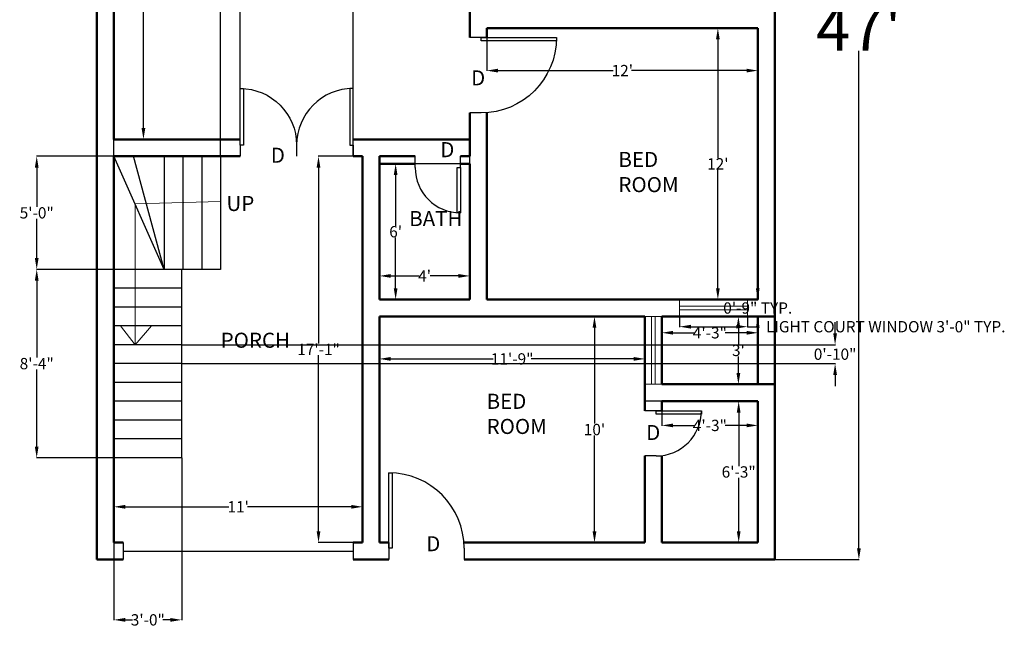
# Model space of a CAD drawing. Units: inches. Extents: x -251 to 272, y 511 to 1173.
# Tile 1 of 2: x -251 to 272, y 511 to 834. Entities that reach past the tile are written whole.
import ezdxf

# ---------------------------------------------------------------- set-up
doc = ezdxf.new("R2010")
doc.units = ezdxf.units.IN
doc.header["$MEASUREMENT"] = 0
doc.layers.get('0').update_dxf_attribs({"color": 3})
for name, color, linetype, lineweight in [('A-ANNO-SYMB', 20, 'Continuous', 18), ('A-AREA-IDEN', 20, 'Continuous', 25), ('A-FLOR', 7, 'Continuous', 25), ('A-WALL', 7, 'Continuous', 50), ('dim', 2, 'Continuous', 18), ('door', 1, 'Continuous', 25), ('stair', 94, 'Continuous', 25), ('text', 20, 'Continuous', 18), ('window', 6, 'Continuous', 18)]:
    doc.layers.add(name, color=color, linetype=linetype, lineweight=lineweight)
doc.styles.get("Standard").update_dxf_attribs({"font": 'arial.ttf'})
doc.dimstyles.get("Standard").update_dxf_attribs({"dimtxt": 6, "dimasz": 6, "dimexe": 0.18, "dimexo": 0.0625, "dimgap": 0.09, "dimtad": 0, "dimtih": 1, "dimtoh": 1, "dimdec": 0, "dimzin": 0, "dimdsep": 46, "dimlunit": 3, "dimtxsty": 'Standard', "dimcen": 0.09, "dimadec": 0, "dimazin": 0, "dimtfac": 1, "dimtdec": 0, "dimtofl": 0, "dimtmove": 0, "dimatfit": 3, "dimfxl": 1, "dimtolj": 1, "dimtzin": 0, "dimarcsym": 0})

# ---------------------------------------------------------------- blocks, each defined once
blk = doc.blocks.new('*U18')
for p, q in [((0, 0), (0, 6)), ((40, 0), (40, 6))]:
    blk.add_line(p, q)
blk.add_lwpolyline([(0, 0), (0, -40), (1.75, -40), (1.75, 0)], close=True)
blk.add_arc((0, 0), 40, 270, 0)
blk = doc.blocks.new('*D21')
at = {"layer": 'Defpoints', "color": 0, "transparency": 16777216}
for p in [(141.31, 829.09), (120.04, 685.09), (141.31, 685.09)]:
    blk.add_point(p, dxfattribs=at)
at = {"layer": 'dim', "color": 0, "lineweight": -2, "transparency": 16777216}
for p, q in [((141.25, 829.09), (119.86, 829.09)), ((120.04, 823.09), (120.04, 760.19)), ((120.04, 691.09), (120.04, 753.99)), ((141.25, 685.09), (119.86, 685.09))]:
    blk.add_line(p, q, dxfattribs=at)
at = {"layer": 'dim', "color": 0, "transparency": 16777216}
for points in [[(119.04, 823.09), (121.04, 823.09), (120.04, 829.09)], [(119.04, 691.09), (121.04, 691.09), (120.04, 685.09)]]:
    blk.add_solid(points, dxfattribs=at)
at = {"layer": 'dim', "color": 0, "transparency": 16777216, "insert": (120.04, 757.09), "char_height": 6, "attachment_point": 5}
blk.add_mtext("\\A1;12'", dxfattribs=at)
blk = doc.blocks.new('*D22')
at = {"layer": 'Defpoints', "color": 0, "transparency": 16777216}
for p in [(-2.69, 829.09), (141.31, 829.09), (-2.69, 806.58)]:
    blk.add_point(p, dxfattribs=at)
at = {"layer": 'dim', "color": 0, "lineweight": -2, "transparency": 16777216}
for p, q in [((-2.69, 829.02), (-2.69, 806.4)), ((141.31, 829.02), (141.31, 806.4)), ((3.31, 806.58), (64.41, 806.58)), ((135.31, 806.58), (74.21, 806.58))]:
    blk.add_line(p, q, dxfattribs=at)
at = {"layer": 'dim', "color": 0, "transparency": 16777216}
for points in [[(3.31, 807.58), (3.31, 805.58), (-2.69, 806.58)], [(135.31, 807.58), (135.31, 805.58), (141.31, 806.58)]]:
    blk.add_solid(points, dxfattribs=at)
at = {"layer": 'dim', "color": 0, "transparency": 16777216, "insert": (69.31, 806.58), "char_height": 6, "attachment_point": 5}
blk.add_mtext("\\A1;12'", dxfattribs=at)
blk = doc.blocks.new('*U23')
for p, q in [((0, 0), (0, -6)), ((24, 0), (24, -6))]:
    blk.add_line(p, q)
blk.add_lwpolyline([(0, 0), (0, 24), (1.75, 24), (1.75, 0)], close=True)
blk.add_arc((0, 0), 24, 0, 90)
blk = doc.blocks.new('*U24')
for p, q in [((-24, 0), (-24, 6)), ((0, 0), (0, 6))]:
    blk.add_line(p, q)
blk.add_lwpolyline([(0, 0), (0, -24), (-1.75, -24), (-1.75, 0)], close=True)
blk.add_arc((0, 0), 24, 180, 270)
blk = doc.blocks.new('*D25')
at = {"layer": 'Defpoints', "color": 0, "transparency": 16777216}
for p in [(-14.19, 757.09), (-51.07, 685.09), (-11.69, 685.09)]:
    blk.add_point(p, dxfattribs=at)
at = {"layer": 'dim', "color": 0, "lineweight": -2, "transparency": 16777216}
for p, q in [((-14.25, 757.09), (-51.25, 757.09)), ((-51.07, 751.09), (-51.07, 724.24)), ((-51.07, 691.09), (-51.07, 717.93)), ((-11.75, 685.09), (-51.25, 685.09))]:
    blk.add_line(p, q, dxfattribs=at)
at = {"layer": 'dim', "color": 0, "transparency": 16777216}
for points in [[(-52.07, 751.09), (-50.07, 751.09), (-51.07, 757.09)], [(-52.07, 691.09), (-50.07, 691.09), (-51.07, 685.09)]]:
    blk.add_solid(points, dxfattribs=at)
at = {"layer": 'dim', "color": 0, "transparency": 16777216, "insert": (-51.07, 721.09), "char_height": 6, "attachment_point": 5}
blk.add_mtext("\\A1;6'", dxfattribs=at)
blk = doc.blocks.new('*D26')
at = {"layer": 'Defpoints', "color": 0, "transparency": 16777216}
for p in [(-11.69, 697.62), (-59.69, 685.09), (-11.69, 685.09)]:
    blk.add_point(p, dxfattribs=at)
at = {"layer": 'dim', "color": 0, "lineweight": -2, "transparency": 16777216}
for p, q in [((-59.69, 685.15), (-59.69, 697.8)), ((-53.69, 697.62), (-38.66, 697.62)), ((-17.69, 697.62), (-32.72, 697.62)), ((-11.69, 685.15), (-11.69, 697.8))]:
    blk.add_line(p, q, dxfattribs=at)
at = {"layer": 'dim', "color": 0, "transparency": 16777216}
for points in [[(-53.69, 698.62), (-53.69, 696.62), (-59.69, 697.62)], [(-17.69, 698.62), (-17.69, 696.62), (-11.69, 697.62)]]:
    blk.add_solid(points, dxfattribs=at)
at = {"layer": 'dim', "color": 0, "transparency": 16777216, "insert": (-35.69, 697.62), "char_height": 6, "attachment_point": 5}
blk.add_mtext("\\A1;4'", dxfattribs=at)
blk = doc.blocks.new('*D27')
at = {"layer": 'Defpoints', "color": 0, "transparency": 16777216}
for p in [(141.31, 676.09), (130.96, 640.09), (141.31, 640.09)]:
    blk.add_point(p, dxfattribs=at)
at = {"layer": 'dim', "color": 0, "lineweight": -2, "transparency": 16777216}
for p, q in [((141.25, 676.09), (130.78, 676.09)), ((130.96, 670.09), (130.96, 661.24)), ((130.96, 646.09), (130.96, 654.93)), ((141.25, 640.09), (130.78, 640.09))]:
    blk.add_line(p, q, dxfattribs=at)
at = {"layer": 'dim', "color": 0, "transparency": 16777216}
for points in [[(129.96, 670.09), (131.96, 670.09), (130.96, 676.09)], [(129.96, 646.09), (131.96, 646.09), (130.96, 640.09)]]:
    blk.add_solid(points, dxfattribs=at)
at = {"layer": 'dim', "color": 0, "transparency": 16777216, "insert": (130.96, 658.09), "char_height": 6, "attachment_point": 5}
blk.add_mtext("\\A1;3'", dxfattribs=at)
blk = doc.blocks.new('*D28')
at = {"layer": 'Defpoints', "color": 0, "transparency": 16777216}
for p in [(90.31, 676.09), (141.31, 676.09), (141.31, 667.45)]:
    blk.add_point(p, dxfattribs=at)
at = {"layer": 'dim', "color": 0, "lineweight": -2, "transparency": 16777216}
for p, q in [((90.31, 676.02), (90.31, 667.27)), ((141.31, 676.02), (141.31, 667.27)), ((96.31, 667.45), (107.63, 667.45)), ((135.31, 667.45), (124, 667.45))]:
    blk.add_line(p, q, dxfattribs=at)
at = {"layer": 'dim', "color": 0, "transparency": 16777216}
for points in [[(96.31, 668.45), (96.31, 666.45), (90.31, 667.45)], [(135.31, 668.45), (135.31, 666.45), (141.31, 667.45)]]:
    blk.add_solid(points, dxfattribs=at)
at = {"layer": 'dim', "color": 0, "transparency": 16777216, "insert": (115.81, 667.45), "char_height": 6, "attachment_point": 5}
blk.add_mtext('\\A1;4\'-3"', dxfattribs=at)
blk = doc.blocks.new('*D29')
at = {"layer": 'Defpoints', "color": 0, "transparency": 16777216}
for p in [(141.31, 631.09), (131.11, 556.09), (141.31, 556.09)]:
    blk.add_point(p, dxfattribs=at)
at = {"layer": 'dim', "color": 0, "lineweight": -2, "transparency": 16777216}
for p, q in [((141.25, 631.09), (130.93, 631.09)), ((131.11, 625.09), (131.11, 596.74)), ((131.11, 562.09), (131.11, 590.43)), ((141.25, 556.09), (130.93, 556.09))]:
    blk.add_line(p, q, dxfattribs=at)
at = {"layer": 'dim', "color": 0, "transparency": 16777216}
for points in [[(130.11, 625.09), (132.11, 625.09), (131.11, 631.09)], [(130.11, 562.09), (132.11, 562.09), (131.11, 556.09)]]:
    blk.add_solid(points, dxfattribs=at)
at = {"layer": 'dim', "color": 0, "transparency": 16777216, "insert": (131.11, 593.59), "char_height": 6, "attachment_point": 5}
blk.add_mtext('\\A1;6\'-3"', dxfattribs=at)
blk = doc.blocks.new('*D30')
at = {"layer": 'Defpoints', "color": 0, "transparency": 16777216}
for p in [(90.31, 631.09), (141.31, 631.09), (141.31, 618.28)]:
    blk.add_point(p, dxfattribs=at)
at = {"layer": 'dim', "color": 0, "lineweight": -2, "transparency": 16777216}
for p, q in [((90.31, 631.02), (90.31, 618.1)), ((141.31, 631.02), (141.31, 618.1)), ((96.31, 618.28), (107.63, 618.28)), ((135.31, 618.28), (124, 618.28))]:
    blk.add_line(p, q, dxfattribs=at)
at = {"layer": 'dim', "color": 0, "transparency": 16777216}
for points in [[(96.31, 619.28), (96.31, 617.28), (90.31, 618.28)], [(135.31, 619.28), (135.31, 617.28), (141.31, 618.28)]]:
    blk.add_solid(points, dxfattribs=at)
at = {"layer": 'dim', "color": 0, "transparency": 16777216, "insert": (115.81, 618.28), "char_height": 6, "attachment_point": 5}
blk.add_mtext('\\A1;4\'-3"', dxfattribs=at)
blk = doc.blocks.new('*U8')
for p, q in [((0, 0), (0, -6)), ((40, 0), (40, -6))]:
    blk.add_line(p, q)
blk.add_lwpolyline([(0, 0), (0, 40), (1.75, 40), (1.75, 0)], close=True)
blk.add_arc((0, 0), 40, 0, 90)
blk = doc.blocks.new('*D31')
at = {"layer": 'Defpoints', "color": 0, "transparency": 16777216}
for p in [(65.76, 676.09), (54.53, 556.09), (65.76, 556.09)]:
    blk.add_point(p, dxfattribs=at)
at = {"layer": 'dim', "color": 0, "lineweight": -2, "transparency": 16777216}
for p, q in [((65.7, 676.09), (54.35, 676.09)), ((54.53, 670.09), (54.53, 619.24)), ((54.53, 562.09), (54.53, 612.93)), ((65.7, 556.09), (54.35, 556.09))]:
    blk.add_line(p, q, dxfattribs=at)
at = {"layer": 'dim', "color": 0, "transparency": 16777216}
for points in [[(53.53, 670.09), (55.53, 670.09), (54.53, 676.09)], [(53.53, 562.09), (55.53, 562.09), (54.53, 556.09)]]:
    blk.add_solid(points, dxfattribs=at)
at = {"layer": 'dim', "color": 0, "transparency": 16777216, "insert": (54.53, 616.09), "char_height": 6, "attachment_point": 5}
blk.add_mtext("\\A1;10'", dxfattribs=at)
blk = doc.blocks.new('*D32')
at = {"layer": 'Defpoints', "color": 0, "transparency": 16777216}
for p in [(-59.69, 676.09), (81.31, 676.09), (81.31, 653.59)]:
    blk.add_point(p, dxfattribs=at)
at = {"layer": 'dim', "color": 0, "lineweight": -2, "transparency": 16777216}
for p, q in [((-59.69, 676.02), (-59.69, 653.41)), ((81.31, 676.02), (81.31, 653.41)), ((-53.69, 653.59), (0.7, 653.59)), ((75.31, 653.59), (20.93, 653.59))]:
    blk.add_line(p, q, dxfattribs=at)
at = {"layer": 'dim', "color": 0, "transparency": 16777216}
for points in [[(-53.69, 654.59), (-53.69, 652.59), (-59.69, 653.59)], [(75.31, 654.59), (75.31, 652.59), (81.31, 653.59)]]:
    blk.add_solid(points, dxfattribs=at)
at = {"layer": 'dim', "color": 0, "transparency": 16777216, "insert": (10.81, 653.59), "char_height": 6, "attachment_point": 5}
blk.add_mtext('\\A1;11\'-9"', dxfattribs=at)
blk = doc.blocks.new('*U33')
for p, q in [((-30, 0), (-30, -6)), ((0, 0), (0, -6))]:
    blk.add_line(p, q)
blk.add_lwpolyline([(0, 0), (0, 30), (-1.75, 30), (-1.75, 0)], close=True)
blk.add_arc((0, 0), 30, 90, 180)
blk = doc.blocks.new('*D34')
at = {"layer": 'Defpoints', "color": 0, "transparency": 16777216}
for p in [(-71.19, 761.09), (-92.03, 556.09), (-71.19, 556.09)]:
    blk.add_point(p, dxfattribs=at)
at = {"layer": 'dim', "color": 0, "lineweight": -2, "transparency": 16777216}
for p, q in [((-71.25, 761.09), (-92.21, 761.09)), ((-92.03, 755.09), (-92.03, 661.69)), ((-92.03, 562.09), (-92.03, 655.49)), ((-71.25, 556.09), (-92.21, 556.09))]:
    blk.add_line(p, q, dxfattribs=at)
at = {"layer": 'dim', "color": 0, "transparency": 16777216}
for points in [[(-93.03, 755.09), (-91.03, 755.09), (-92.03, 761.09)], [(-93.03, 562.09), (-91.03, 562.09), (-92.03, 556.09)]]:
    blk.add_solid(points, dxfattribs=at)
at = {"layer": 'dim', "color": 0, "transparency": 16777216, "insert": (-92.03, 658.59), "char_height": 6, "attachment_point": 5}
blk.add_mtext('\\A1;17\'-1"', dxfattribs=at)
blk = doc.blocks.new('*D35')
at = {"layer": 'Defpoints', "color": 0, "transparency": 16777216}
for p in [(-200.69, 583.2), (-68.69, 583.2), (-68.69, 575.09)]:
    blk.add_point(p, dxfattribs=at)
at = {"layer": 'dim', "color": 0, "lineweight": -2, "transparency": 16777216}
for p, q in [((-200.69, 583.14), (-200.69, 574.91)), ((-68.69, 583.14), (-68.69, 574.91)), ((-194.69, 575.09), (-139.59, 575.09)), ((-74.69, 575.09), (-129.79, 575.09))]:
    blk.add_line(p, q, dxfattribs=at)
at = {"layer": 'dim', "color": 0, "transparency": 16777216}
for points in [[(-194.69, 576.09), (-194.69, 574.09), (-200.69, 575.09)], [(-74.69, 576.09), (-74.69, 574.09), (-68.69, 575.09)]]:
    blk.add_solid(points, dxfattribs=at)
at = {"layer": 'dim', "color": 0, "transparency": 16777216, "insert": (-134.69, 575.09), "char_height": 6, "attachment_point": 5}
blk.add_mtext("\\A1;11'", dxfattribs=at)
blk = doc.blocks.new('*D36')
at = {"layer": 'Defpoints', "color": 0, "transparency": 16777216}
for p in [(-200.69, 914.09), (-200.69, 770.09), (-185.02, 770.09)]:
    blk.add_point(p, dxfattribs=at)
at = {"layer": 'dim', "color": 0, "lineweight": -2, "transparency": 16777216}
for p, q in [((-200.63, 914.09), (-184.84, 914.09)), ((-185.02, 908.09), (-185.02, 845.19)), ((-185.02, 776.09), (-185.02, 838.99)), ((-200.63, 770.09), (-184.84, 770.09))]:
    blk.add_line(p, q, dxfattribs=at)
at = {"layer": 'dim', "color": 0, "transparency": 16777216}
for points in [[(-186.02, 908.09), (-184.02, 908.09), (-185.02, 914.09)], [(-186.02, 776.09), (-184.02, 776.09), (-185.02, 770.09)]]:
    blk.add_solid(points, dxfattribs=at)
at = {"layer": 'dim', "color": 0, "transparency": 16777216, "insert": (-185.02, 842.09), "char_height": 6, "attachment_point": 5}
blk.add_mtext("\\A1;12'", dxfattribs=at)
blk = doc.blocks.new('*D38')
at = {"layer": 'Defpoints', "color": 0, "transparency": 16777216}
for p in [(150.31, 1111.09), (150.31, 547.09), (194.95, 547.09)]:
    blk.add_point(p, dxfattribs=at)
at = {"layer": 'dim', "color": 0, "lineweight": -2, "transparency": 16777216}
for p, q in [((150.37, 1111.09), (195.13, 1111.09)), ((194.95, 1105.09), (194.95, 841.18)), ((194.95, 553.09), (194.95, 817)), ((150.37, 547.09), (195.13, 547.09))]:
    blk.add_line(p, q, dxfattribs=at)
at = {"layer": 'dim', "color": 0, "transparency": 16777216}
for points in [[(193.95, 1105.09), (195.95, 1105.09), (194.95, 1111.09)], [(193.95, 553.09), (195.95, 553.09), (194.95, 547.09)]]:
    blk.add_solid(points, dxfattribs=at)
at = {"layer": 'dim', "color": 0, "transparency": 16777216, "insert": (194.95, 829.09), "char_height": 6, "attachment_point": 5}
blk.add_mtext("\\A1;{\\H4x;47'}", dxfattribs=at)
blk = doc.blocks.new('WIN-36IN-LIGHTCOURT')
for p, q in [((0, 9), (0, 0)), ((0, 5.5), (36.12, 5.5)), ((36.12, 9), (36.12, 0)), ((0, 3.5), (36.12, 3.5))]:
    blk.add_line(p, q)
blk = doc.blocks.new('*D41')
at = {"layer": 'Defpoints', "color": 0, "transparency": 16777216}
for p in [(99.7, 676.09), (135.82, 676.09), (135.82, 670.67)]:
    blk.add_point(p, dxfattribs=at)
at = {"layer": 'dim', "color": 0, "lineweight": -2, "transparency": 16777216}
for p, q in [((99.7, 676.02), (99.7, 670.49)), ((135.82, 676.02), (135.82, 670.49)), ((105.7, 670.67), (129.82, 670.67)), ((135.82, 670.67), (141.82, 670.67))]:
    blk.add_line(p, q, dxfattribs=at)
at = {"layer": 'dim', "color": 0, "transparency": 16777216}
for points in [[(105.7, 671.67), (105.7, 669.67), (99.7, 670.67)], [(129.82, 671.67), (129.82, 669.67), (135.82, 670.67)]]:
    blk.add_solid(points, dxfattribs=at)
at = {"layer": 'dim', "color": 0, "transparency": 16777216, "insert": (209.19, 670.67), "char_height": 6, "attachment_point": 5}
blk.add_mtext('\\A1;LIGHT COURT WINDOW 3\'-0" TYP.', dxfattribs=at)
blk = doc.blocks.new('*D42')
at = {"layer": 'Defpoints', "color": 0, "transparency": 16777216}
for p in [(135.82, 685.09), (141.24, 685.09), (135.82, 676.09)]:
    blk.add_point(p, dxfattribs=at)
at = {"layer": 'dim', "color": 0, "lineweight": -2, "transparency": 16777216}
for p, q in [((141.24, 691.09), (141.24, 697.09)), ((135.89, 685.09), (141.42, 685.09)), ((135.89, 676.09), (141.42, 676.09)), ((141.24, 670.09), (141.24, 664.09))]:
    blk.add_line(p, q, dxfattribs=at)
at = {"layer": 'dim', "color": 0, "transparency": 16777216}
for points in [[(140.24, 691.09), (142.24, 691.09), (141.24, 685.09)], [(140.24, 670.09), (142.24, 670.09), (141.24, 676.09)]]:
    blk.add_solid(points, dxfattribs=at)
at = {"layer": 'dim', "color": 0, "transparency": 16777216, "insert": (141.24, 680.59), "char_height": 6, "attachment_point": 5}
blk.add_mtext('\\A1;0\'-9" TYP.', dxfattribs=at)
blk = doc.blocks.new('*D43')
at = {"layer": 'Defpoints', "color": 0, "transparency": 16777216}
for p in [(-200.69, 601.09), (-164.69, 601.09), (-164.69, 515.09)]:
    blk.add_point(p, dxfattribs=at)
at = {"layer": 'dim', "color": 0, "lineweight": -2, "transparency": 16777216}
for p, q in [((-200.69, 601.02), (-200.69, 514.91)), ((-164.69, 601.02), (-164.69, 514.91)), ((-194.69, 515.09), (-190.75, 515.09)), ((-170.69, 515.09), (-174.63, 515.09))]:
    blk.add_line(p, q, dxfattribs=at)
at = {"layer": 'dim', "color": 0, "transparency": 16777216}
for points in [[(-194.69, 516.09), (-194.69, 514.09), (-200.69, 515.09)], [(-170.69, 516.09), (-170.69, 514.09), (-164.69, 515.09)]]:
    blk.add_solid(points, dxfattribs=at)
at = {"layer": 'dim', "color": 0, "transparency": 16777216, "insert": (-182.69, 515.09), "char_height": 6, "attachment_point": 5}
blk.add_mtext('\\A1;3\'-0"', dxfattribs=at)
blk = doc.blocks.new('*D44')
at = {"layer": 'Defpoints', "color": 0, "transparency": 16777216}
for p in [(-241.69, 701.09), (-200.69, 701.09), (-200.69, 601.09)]:
    blk.add_point(p, dxfattribs=at)
at = {"layer": 'dim', "color": 0, "lineweight": -2, "transparency": 16777216}
for p, q in [((-200.75, 701.09), (-241.87, 701.09)), ((-241.69, 695.09), (-241.69, 654.24)), ((-241.69, 607.09), (-241.69, 647.93)), ((-200.75, 601.09), (-241.87, 601.09))]:
    blk.add_line(p, q, dxfattribs=at)
at = {"layer": 'dim', "color": 0, "transparency": 16777216}
for points in [[(-242.69, 695.09), (-240.69, 695.09), (-241.69, 701.09)], [(-242.69, 607.09), (-240.69, 607.09), (-241.69, 601.09)]]:
    blk.add_solid(points, dxfattribs=at)
at = {"layer": 'dim', "color": 0, "transparency": 16777216, "insert": (-241.69, 651.09), "char_height": 6, "attachment_point": 5}
blk.add_mtext('\\A1;8\'-4"', dxfattribs=at)
blk = doc.blocks.new('*D45')
at = {"layer": 'Defpoints', "color": 0, "transparency": 16777216}
for p in [(-164.688189, 661.087339), (182.311811, 661.087339), (-164.688189, 651.087339)]:
    blk.add_point(p, dxfattribs=at)
at = {"layer": 'dim', "color": 0, "lineweight": -2, "transparency": 16777216}
for p, q in [((182.311811, 667.087339), (182.311811, 673.087339)), ((-164.625689, 661.087339), (182.491811, 661.087339)), ((-164.625689, 651.087339), (182.491811, 651.087339)), ((182.311811, 645.087339), (182.311811, 639.087339))]:
    blk.add_line(p, q, dxfattribs=at)
at = {"layer": 'dim', "color": 0, "transparency": 16777216}
for points in [[(181.311811, 667.087339), (183.311811, 667.087339), (182.311811, 661.087339)], [(181.311811, 645.087339), (183.311811, 645.087339), (182.311811, 651.087339)]]:
    blk.add_solid(points, dxfattribs=at)
at = {"layer": 'dim', "color": 0, "transparency": 16777216, "insert": (182.311811, 656.087339), "char_height": 6, "attachment_point": 5}
blk.add_mtext('\\A1;0\'-10"', dxfattribs=at)
blk = doc.blocks.new('*D46')
at = {"layer": 'Defpoints', "color": 0, "transparency": 16777216}
for p in [(-241.69, 761.09), (-200.69, 761.09), (-200.69, 701.09)]:
    blk.add_point(p, dxfattribs=at)
at = {"layer": 'dim', "color": 0, "lineweight": -2, "transparency": 16777216}
for p, q in [((-200.75, 761.09), (-241.87, 761.09)), ((-241.69, 755.09), (-241.69, 734.24)), ((-241.69, 707.09), (-241.69, 727.93)), ((-200.75, 701.09), (-241.87, 701.09))]:
    blk.add_line(p, q, dxfattribs=at)
at = {"layer": 'dim', "color": 0, "transparency": 16777216}
for points in [[(-242.69, 755.09), (-240.69, 755.09), (-241.69, 761.09)], [(-242.69, 707.09), (-240.69, 707.09), (-241.69, 701.09)]]:
    blk.add_solid(points, dxfattribs=at)
at = {"layer": 'dim', "color": 0, "transparency": 16777216, "insert": (-241.69, 731.09), "char_height": 6, "attachment_point": 5}
blk.add_mtext('\\A1;5\'-0"', dxfattribs=at)
blk = doc.blocks.new('*D47')
at = {"layer": 'Defpoints', "color": 0, "transparency": 16777216}
for p in [(-144.01, 1143.09), (-200.69, 761.09), (-144.01, 761.09)]:
    blk.add_point(p, dxfattribs=at)
at = {"layer": 'dim', "color": 0, "lineweight": -2, "transparency": 16777216}
for p, q in [((-200.69, 761.15), (-200.69, 1143.27)), ((-194.69, 1143.09), (-187.52, 1143.09)), ((-150.01, 1143.09), (-157.17, 1143.09)), ((-144.01, 761.15), (-144.01, 1143.27))]:
    blk.add_line(p, q, dxfattribs=at)
at = {"layer": 'dim', "color": 0, "transparency": 16777216}
for points in [[(-194.69, 1144.09), (-194.69, 1142.09), (-200.69, 1143.09)], [(-150.01, 1144.09), (-150.01, 1142.09), (-144.01, 1143.09)]]:
    blk.add_solid(points, dxfattribs=at)
at = {"layer": 'dim', "color": 0, "transparency": 16777216, "insert": (-172.35, 1143.09), "char_height": 6, "attachment_point": 5}
blk.add_mtext('\\A1;4\'-8 1/2"', dxfattribs=at)
blk = doc.blocks.new('*D49')
at = {"layer": 'Defpoints', "color": 0, "transparency": 16777216}
for p in [(-73.69, 1143.09), (-133.69, 770.09), (-73.69, 770.09)]:
    blk.add_point(p, dxfattribs=at)
at = {"layer": 'dim', "color": 0, "lineweight": -2, "transparency": 16777216}
for p, q in [((-133.69, 770.15), (-133.69, 1143.27)), ((-127.69, 1143.09), (-111.75, 1143.09)), ((-79.69, 1143.09), (-95.62, 1143.09)), ((-73.69, 770.15), (-73.69, 1143.27))]:
    blk.add_line(p, q, dxfattribs=at)
at = {"layer": 'dim', "color": 0, "transparency": 16777216}
for points in [[(-127.69, 1144.09), (-127.69, 1142.09), (-133.69, 1143.09)], [(-79.69, 1144.09), (-79.69, 1142.09), (-73.69, 1143.09)]]:
    blk.add_solid(points, dxfattribs=at)
at = {"layer": 'dim', "color": 0, "transparency": 16777216, "insert": (-103.69, 1143.09), "char_height": 6, "attachment_point": 5}
blk.add_mtext('\\A1;5\'-0"', dxfattribs=at)
blk = doc.blocks.new('*D50')
at = {"layer": 'Defpoints', "color": 0, "transparency": 16777216}
for p in [(-133.69, 1143.09), (-200.69, 770.09), (-133.69, 770.09)]:
    blk.add_point(p, dxfattribs=at)
at = {"layer": 'dim', "color": 0, "lineweight": -2, "transparency": 16777216}
for p, q in [((-200.69, 770.15), (-200.69, 1143.27)), ((-194.69, 1143.09), (-175.25, 1143.09)), ((-139.69, 1143.09), (-159.12, 1143.09)), ((-133.69, 770.15), (-133.69, 1143.27))]:
    blk.add_line(p, q, dxfattribs=at)
at = {"layer": 'dim', "color": 0, "transparency": 16777216}
for points in [[(-194.69, 1144.09), (-194.69, 1142.09), (-200.69, 1143.09)], [(-139.69, 1144.09), (-139.69, 1142.09), (-133.69, 1143.09)]]:
    blk.add_solid(points, dxfattribs=at)
at = {"layer": 'dim', "color": 0, "transparency": 16777216, "insert": (-167.19, 1143.09), "char_height": 6, "attachment_point": 5}
blk.add_mtext('\\A1;5\'-7"', dxfattribs=at)

msp = doc.modelspace()

# ---------------------------------------------------------------- linework, layer by layer
at = {"layer": 'A-ANNO-SYMB'}
for p, q in [((-144.01, 737.05), (-189.47, 735.87)), ((-189.47, 735.87), (-189.47, 661.09)), ((-189.47, 661.09), (-197.2, 671.09)), ((-197.2, 671.09), (-180.78, 671.09)), ((-180.78, 671.09), (-189.47, 661.09))]:
    msp.add_line(p, q, dxfattribs=at)
at = {"layer": 'A-FLOR'}
for p, q in [((-195.69, 556.09), (-195.69, 547.09)), ((-73.69, 556.09), (-73.69, 547.09)), ((-195.69, 551.59), (-73.69, 551.59))]:
    msp.add_line(p, q, dxfattribs=at)
at = {"layer": 'A-WALL'}
for p, q in [((-209.69, 547.09), (-209.69, 1111.09)), ((150.31, 1111.09), (150.31, 547.09)), ((-200.69, 770.09), (-200.69, 914.09)), ((-200.69, 770.09), (-200.69, 914.09)), ((-11.69, 843.09), (-11.69, 829.09)), ((-11.69, 843.09), (-11.69, 824.09)), ((-11.69, 829.09), (-11.69, 824.09)), ((-2.69, 829.09), (141.31, 829.09)), ((141.31, 829.09), (-2.69, 829.09)), ((-2.69, 829.09), (-2.69, 824.09)), ((141.31, 829.09), (141.31, 685.09)), ((141.31, 685.09), (141.31, 829.09)), ((-11.69, 784.09), (-11.69, 766.09)), ((-11.69, 784.09), (-11.69, 761.09)), ((-2.69, 784.2), (-2.69, 685.09)), ((-133.69, 770.09), (-200.69, 770.09)), ((-103.54, 770.09), (-103.84, 770.09)), ((-11.69, 770.09), (-73.69, 770.09)), ((-200.69, 556.09), (-200.69, 761.09)), ((-133.69, 761.09), (-200.69, 761.09)), ((-68.69, 761.09), (-73.69, 761.09)), ((-68.69, 761.09), (-68.69, 685.09)), ((-59.69, 761.09), (-59.69, 685.09)), ((-40.69, 761.09), (-59.69, 761.09)), ((-11.69, 761.09), (-16.69, 761.09)), ((-40.5, 757.09), (-59.69, 757.09)), ((-11.69, 757.09), (-16.69, 757.09)), ((-11.69, 685.09), (-11.69, 757.09)), ((-11.69, 757.09), (-11.69, 685.09)), ((-68.69, 556.09), (-68.69, 685.09)), ((-59.69, 685.09), (-11.69, 685.09)), ((-59.69, 685.09), (-11.69, 685.09)), ((-2.69, 685.09), (141.31, 685.09)), ((-59.69, 676.09), (81.31, 676.09)), ((-59.69, 676.09), (-59.69, 556.09)), ((81.31, 676.09), (81.31, 631.09)), ((150.31, 676.09), (90.31, 676.09)), ((90.31, 676.09), (90.31, 640.09)), ((90.31, 676.09), (141.31, 676.09)), ((141.31, 676.09), (141.31, 640.09)), ((141.31, 640.09), (141.31, 676.09)), ((90.31, 640.09), (150.31, 640.09)), ((81.31, 631.09), (81.31, 626.09)), ((90.31, 631.09), (141.31, 631.09)), ((141.31, 631.09), (90.31, 631.09)), ((90.31, 631.09), (90.31, 626.09)), ((141.31, 631.09), (141.31, 556.09)), ((141.31, 556.09), (141.31, 631.09)), ((81.31, 602.09), (81.31, 556.09)), ((90.31, 602.28), (90.31, 556.09)), ((-195.69, 556.09), (-200.69, 556.09)), ((-68.69, 556.09), (-73.69, 556.09)), ((-54.69, 556.09), (-59.69, 556.09)), ((81.31, 556.09), (-14.8, 556.09)), ((141.31, 556.09), (90.31, 556.09)), ((-195.69, 547.09), (-209.69, 547.09)), ((-54.69, 547.09), (-73.69, 547.09)), ((150.31, 547.09), (-14.69, 547.09))]:
    msp.add_line(p, q, dxfattribs=at)
at = {"layer": 'door'}
for p, q in [((-2.69, 824.09), (-11.69, 824.09)), ((-73.69, 761.09), (-73.69, 770.09)), ((-11.69, 757.09), (-11.69, 761.09)), ((90.31, 631.09), (81.31, 631.09)), ((90.31, 626.09), (81.31, 626.09)), ((-54.69, 556.09), (-54.69, 547.09))]:
    msp.add_line(p, q, dxfattribs=at)
at = {"layer": 'stair'}
for p, q in [((-174.01, 701.09), (-200.69, 761.09)), ((-174.01, 701.09), (-190.37, 761.09)), ((-174.01, 761.09), (-174.01, 701.09)), ((-164.01, 761.09), (-164.01, 701.09)), ((-154.01, 761.09), (-154.01, 701.09)), ((-144.01, 761.09), (-144.01, 701.09)), ((-144.01, 701.09), (-200.69, 701.09)), ((-164.69, 601.09), (-164.69, 701.09)), ((-164.69, 691.09), (-200.69, 691.09)), ((-164.69, 681.09), (-200.69, 681.09)), ((-164.69, 671.09), (-200.69, 671.09)), ((-164.69, 661.09), (-200.69, 661.09)), ((-164.69, 651.09), (-200.69, 651.09)), ((-164.69, 641.09), (-200.69, 641.09)), ((-164.69, 631.09), (-200.69, 631.09)), ((-164.69, 621.09), (-200.69, 621.09)), ((-164.69, 611.09), (-200.69, 611.09)), ((-164.69, 601.09), (-200.69, 601.09))]:
    msp.add_line(p, q, dxfattribs=at)

# ---------------------------------------------------------------- block references
at = {"layer": 'door', "xscale": -1}
for name, p, rotation in [('*U18', (-5.69, 824.09), 90), ('*U33', (-133.69, 767.09), 359.9999999999998)]:
    msp.add_blockref(name, p, dxfattribs=dict(at, rotation=rotation))
at = {"layer": 'door'}
for name, p in [('*U33', (-73.69, 767.09)), ('*U24', (-16.69, 755.09)), ('*U8', (-54.69, 553.09))]:
    msp.add_blockref(name, p, dxfattribs=at)
at = {"layer": 'door', "rotation": 270}
msp.add_blockref('*U23', (87.31, 626.09), dxfattribs=at)
at = {"layer": 'window'}
msp.add_blockref('WIN-36IN-LIGHTCOURT', (99.7, 676.09), dxfattribs=at)
at = {"layer": 'window', "xscale": 0.9966651399995846, "rotation": 89.99999999999976}
msp.add_blockref('WIN-36IN-LIGHTCOURT', (90.31, 640.09), dxfattribs=at)

# ---------------------------------------------------------------- texts
at = {"layer": 'A-AREA-IDEN', "char_height": 8, "attachment_point": 1}
for s, width, insert in [('BED ROOM', 53.8549, (67.23, 763.41)), ('BATH', 12.3166, (-43.88, 732.07)), ('PORCH', 38.6268, (-144.01, 667.48)), ('BED ROOM', 53.8549, (-2.76, 635.08))]:
    msp.add_mtext_dynamic_manual_height_columns(s, width=width, gutter_width=1, heights=[0], dxfattribs=dict(at, insert=insert))
at = {"layer": 'text', "char_height": 8, "attachment_point": 1}
for s, width, heights, insert in [('D', 6.3802, [0], (-11, 806.72)), ('D', 6.3802, [0], (-117.37, 765.67)), ('D', 6.3802, [0], (-27.39, 768.63)), ('UP', 13.872, [0.203], (-140.92, 740.06)), ('D', 6.3802, [0], (81.98, 618.52)), ('D', 6.3802, [0], (-34.84, 559.49))]:
    msp.add_mtext_dynamic_manual_height_columns(s, width=width, gutter_width=1, heights=heights, dxfattribs=dict(at, insert=insert))

# ---------------------------------------------------------------- dimensions: what is measured, and where the dimension line sits
at = {"layer": 'dim'}
for base, p1, p2, override, picture, middle in [((-144.01, 1143.09), (-200.69, 761.09), (-144.01, 761.09), {"dimdec": 1, "dimlfac": 1, "dimrnd": 0, "dimzin": 1, "dimdsep": 46, "dimlunit": 4, "dimfrac": 2}, '*D47', (-172.35, 1143.09)), ((-133.69, 1143.09), (-200.69, 770.09), (-133.69, 770.09), {"dimdec": 1, "dimlfac": 1, "dimrnd": 0, "dimzin": 1, "dimdsep": 46, "dimlunit": 4, "dimfrac": 2}, '*D50', (-167.19, 1143.09)), ((-73.69, 1143.09), (-133.69, 770.09), (-73.69, 770.09), {"dimdec": 1, "dimlfac": 1, "dimrnd": 0, "dimzin": 1, "dimdsep": 46, "dimlunit": 4, "dimfrac": 2}, '*D49', (-103.69, 1143.09)), ((-2.69, 806.58), (141.31, 829.09), (-2.69, 829.09), {"dimclrd": 0, "dimclre": 0, "dimclrt": 0}, '*D22', (69.31, 806.58)), ((-11.69, 697.62), (-59.69, 685.09), (-11.69, 685.09), {"dimclrd": 0, "dimclre": 0, "dimclrt": 0}, '*D26', (-35.69, 697.62)), ((81.31, 653.59), (-59.69, 676.09), (81.31, 676.09), {"dimclrd": 0, "dimclre": 0, "dimclrt": 0}, '*D32', (10.81, 653.59)), ((141.31, 667.45), (90.31, 676.09), (141.31, 676.09), {"dimclrd": 0, "dimclre": 0, "dimclrt": 0}, '*D28', (115.81, 667.45)), ((141.31, 618.28), (90.31, 631.09), (141.31, 631.09), {"dimclrd": 0, "dimclre": 0, "dimclrt": 0}, '*D30', (115.81, 618.28)), ((-164.69, 515.09), (-200.69, 601.09), (-164.69, 601.09), {"dimdec": 1, "dimlfac": 1, "dimrnd": 0, "dimzin": 1, "dimdsep": 46, "dimlunit": 4, "dimfrac": 2}, '*D43', (-182.69, 515.09)), ((-68.69, 575.09), (-200.69, 583.2), (-68.69, 583.2), {"dimclrd": 0, "dimclre": 0, "dimclrt": 0}, '*D35', (-134.69, 575.09))]:
    dim = msp.add_linear_dim(base=base, p1=p1, p2=p2, dimstyle='Standard', override=override, dxfattribs=at)
    dim.commit()
    dim.dimension.update_dxf_attribs({"geometry": picture, "text_midpoint": middle})
for base, p1, p2, text, override, picture, middle in [((194.95, 547.09), (150.31, 1111.09), (150.31, 547.09), '{\\H4x;<>}', {"dimclrd": 0, "dimclre": 0, "dimclrt": 0}, '*D38', (194.95, 829.09)), ((141.24, 685.09), (135.82, 676.09), (135.82, 685.09), '<> TYP.', {"dimdec": 1, "dimlfac": 1, "dimrnd": 0, "dimzin": 1, "dimdsep": 46, "dimlunit": 4, "dimfrac": 2}, '*D42', (141.24, 680.59))]:
    dim = msp.add_linear_dim(base=base, p1=p1, p2=p2, angle=90, text=text, dimstyle='Standard', override=override, dxfattribs=at)
    dim.commit()
    dim.dimension.update_dxf_attribs({"geometry": picture, "text_midpoint": middle})
for base, p1, p2, override, picture, middle in [((-185.02, 770.09), (-200.69, 914.09), (-200.69, 770.09), {"dimclrd": 0, "dimclre": 0, "dimclrt": 0}, '*D36', (-185.02, 842.09)), ((120.04, 685.09), (141.31, 829.09), (141.31, 685.09), {"dimclrd": 0, "dimclre": 0, "dimclrt": 0}, '*D21', (120.04, 757.09)), ((-241.69, 761.09), (-200.69, 701.09), (-200.69, 761.09), {"dimdec": 1, "dimlfac": 1, "dimrnd": 0, "dimzin": 1, "dimdsep": 46, "dimlunit": 4, "dimfrac": 2}, '*D46', (-241.69, 731.09)), ((-92.03, 556.09), (-71.19, 761.09), (-71.19, 556.09), {"dimclrd": 0, "dimclre": 0, "dimclrt": 0}, '*D34', (-92.03, 658.59)), ((-51.07, 685.09), (-14.19, 757.09), (-11.69, 685.09), {"dimclrd": 0, "dimclre": 0, "dimclrt": 0}, '*D25', (-51.07, 721.09)), ((-241.69, 701.09), (-200.69, 601.09), (-200.69, 701.09), {"dimdec": 1, "dimlfac": 1, "dimrnd": 0, "dimzin": 1, "dimdsep": 46, "dimlunit": 4, "dimfrac": 2}, '*D44', (-241.69, 651.09)), ((54.53, 556.09), (65.76, 676.09), (65.76, 556.09), {"dimclrd": 0, "dimclre": 0, "dimclrt": 0}, '*D31', (54.53, 616.09)), ((130.96, 640.09), (141.31, 676.09), (141.31, 640.09), {"dimclrd": 0, "dimclre": 0, "dimclrt": 0}, '*D27', (130.96, 658.09)), ((182.31, 661.09), (-164.69, 651.09), (-164.69, 661.09), {"dimdec": 1, "dimlfac": 1, "dimrnd": 0, "dimzin": 1, "dimdsep": 46, "dimlunit": 4, "dimfrac": 2}, '*D45', (182.31, 656.09)), ((131.11, 556.09), (141.31, 631.09), (141.31, 556.09), {"dimclrd": 0, "dimclre": 0, "dimclrt": 0}, '*D29', (131.11, 593.59))]:
    dim = msp.add_linear_dim(base=base, p1=p1, p2=p2, angle=90, dimstyle='Standard', override=override, dxfattribs=at)
    dim.commit()
    dim.dimension.update_dxf_attribs({"geometry": picture, "text_midpoint": middle})
dim = msp.add_linear_dim(base=(135.82, 670.67), p1=(99.7, 676.09), p2=(135.82, 676.09), text='LIGHT COURT WINDOW <> TYP.', dimstyle='Standard', override={"dimdec": 1, "dimlfac": 1, "dimrnd": 0, "dimzin": 1, "dimdsep": 46, "dimlunit": 4, "dimfrac": 2}, dxfattribs=at)
dim.commit()
dim.dimension.update_dxf_attribs({"geometry": '*D41', "text_midpoint": (209.19, 670.67)})

doc.saveas('drawing.dxf')
